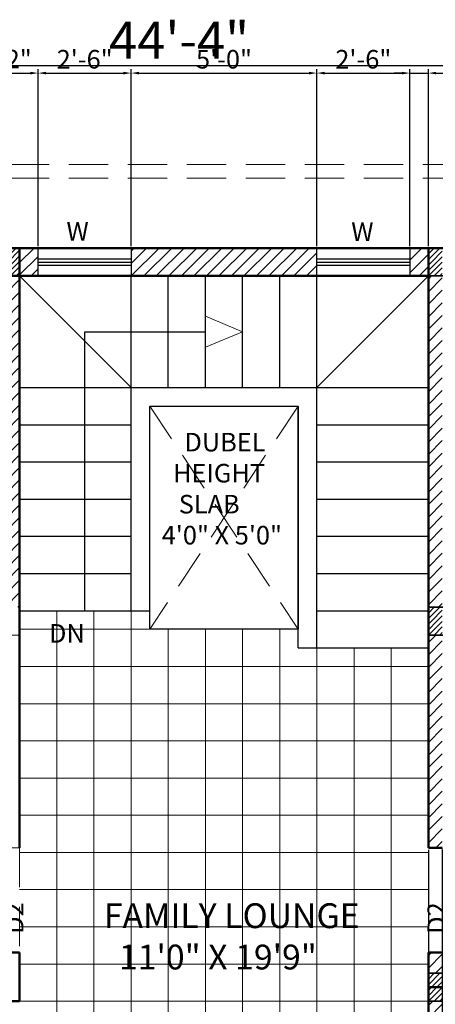
# Model space of a CAD drawing. Units: millimetres. Extents: x 225995 to 227247, y 225507 to 226008.
# Tile 17 of 23: x 226894 to 227029, y 225691 to 226008. Entities that reach past the tile are written whole.
import ezdxf

# ---------------------------------------------------------------- set-up
doc = ezdxf.new("R2010")
doc.units = ezdxf.units.MM
doc.linetypes.add('DASHED', pattern=[19.05, 12.7, -6.35])
for name, color, linetype, lineweight in [('A-ANNO-DIMS', 2, 'Continuous', 18), ('A-ANNO-TEXT', 3, 'Continuous', 18), ('A-AREA-IDEN', 30, 'Continuous', 18), ('A-COLS', 40, 'Continuous', 35), ('A-FLOR-PATT', 8, 'Continuous', 13), ('A-FLOR-STRS', 141, 'Continuous', 25), ('A-FURN', 9, 'Continuous', 18), ('A-GLAZ', 4, 'Continuous', 25), ('A-WALL', 7, 'Continuous', 50), ('A-WALL-OVHD', 1, 'DASHED', 18), ('A-WALL-PATT', 8, 'Continuous', 13)]:
    doc.layers.add(name, color=color, linetype=linetype, lineweight=lineweight)
doc.styles.get("Standard").update_dxf_attribs({"font": 'arial.ttf'})
doc.dimstyles.new('ISO-25', dxfattribs={"dimtxt": 6, "dimasz": 2.5, "dimexe": 1.25, "dimexo": 0.625, "dimtad": 1, "dimdec": 0, "dimlunit": 3, "dimtxsty": 'Standard', "dimcen": 2.5, "dimadec": 0, "dimazin": 0, "dimtfac": 1, "dimtdec": 0, "dimtmove": 0, "dimatfit": 3, "dimfxl": 1, "dimarcsym": 0})
pattern_1 = [(45, (646.0463, 0.931), (-2.020557627, 2.020557627), [])]
pattern_2 = [(45, (646.0463, 0.931), (-0.898025612, 0.898025612), [])]
pattern_3 = [(45, (646.0463, 119.0672), (-0.898025612, 0.898025612), [])]
pattern_4 = [(45, (646.0463, 234.931), (-0.898025612, 0.898025612), [])]
pattern_5 = [(45, (502.0463, 234.931), (-0.898025612, 0.898025612), [])]

# ---------------------------------------------------------------- blocks, each defined once
blk = doc.blocks.new('*D70')
at = {"layer": 'A-ANNO-DIMS', "color": 0, "lineweight": -2, "transparency": 16777216}
for p, q in [((226679.92, 225962.33), (226679.92, 225994.83)), ((227211.92, 225962.33), (227211.92, 225994.83)), ((226682.42, 225993.58), (227209.42, 225993.58))]:
    blk.add_line(p, q, dxfattribs=at)
at = {"layer": 'A-ANNO-DIMS', "color": 0, "transparency": 16777216}
for points in [[(226682.42, 225993.99), (226682.42, 225993.16), (226679.92, 225993.58)], [(227209.42, 225993.99), (227209.42, 225993.16), (227211.92, 225993.58)]]:
    blk.add_solid(points, dxfattribs=at)
at = {"layer": 'Defpoints', "color": 0, "transparency": 16777216}
for p in [(227211.92, 225993.58), (226679.92, 225961.7), (227211.92, 225961.7)]:
    blk.add_point(p, dxfattribs=at)
at = {"layer": 'A-ANNO-DIMS', "color": 0, "transparency": 16777216, "insert": (226945.92, 226000.2), "char_height": 12, "attachment_point": 5}
blk.add_mtext('44\'-4"', dxfattribs=at)
blk = doc.blocks.new('*D115')
at = {"layer": 'A-ANNO-DIMS', "color": 0, "lineweight": -2, "transparency": 16777216}
for p, q in [((227026.42, 225740.58), (227026.42, 225520)), ((227030.92, 225740.58), (227030.92, 225520)), ((227023.92, 225521.25), (227021.42, 225521.25)), ((227026.42, 225521.25), (227030.92, 225521.25)), ((227033.42, 225521.25), (227067.1, 225521.25))]:
    blk.add_line(p, q, dxfattribs=at)
at = {"layer": 'A-ANNO-DIMS', "color": 0, "transparency": 16777216}
for points in [[(227023.92, 225521.67), (227023.92, 225520.84), (227026.42, 225521.25)], [(227033.42, 225521.67), (227033.42, 225520.84), (227030.92, 225521.25)]]:
    blk.add_solid(points, dxfattribs=at)
at = {"layer": 'Defpoints', "color": 0, "transparency": 16777216}
for p in [(227026.42, 225741.2), (227030.92, 225741.2), (227030.92, 225521.25)]:
    blk.add_point(p, dxfattribs=at)
at = {"layer": 'A-ANNO-DIMS', "color": 0, "transparency": 16777216, "insert": (227051.51, 225524.98), "char_height": 6, "attachment_point": 5}
blk.add_mtext('0\'-4 1/2"', dxfattribs=at)
blk = doc.blocks.new('*D117')
at = {"layer": 'A-ANNO-DIMS', "color": 0, "lineweight": -2, "transparency": 16777216}
for p, q in [((226864.05, 225935.33), (226864.05, 225992.4)), ((226866.55, 225991.15), (226897.92, 225991.15)), ((226900.42, 225935.33), (226900.42, 225992.4))]:
    blk.add_line(p, q, dxfattribs=at)
at = {"layer": 'A-ANNO-DIMS', "color": 0, "transparency": 16777216}
for points in [[(226866.55, 225991.57), (226866.55, 225990.74), (226864.05, 225991.15)], [(226897.92, 225991.57), (226897.92, 225990.74), (226900.42, 225991.15)]]:
    blk.add_solid(points, dxfattribs=at)
at = {"layer": 'Defpoints', "color": 0, "transparency": 16777216}
for p in [(226900.42, 225991.15), (226864.05, 225934.7), (226900.42, 225934.7)]:
    blk.add_point(p, dxfattribs=at)
at = {"layer": 'A-ANNO-DIMS', "color": 0, "transparency": 16777216, "insert": (226882.23, 225994.88), "char_height": 6, "attachment_point": 5}
blk.add_mtext('3\'-0 1/2"', dxfattribs=at)
blk = doc.blocks.new('*D118')
at = {"layer": 'A-ANNO-DIMS', "color": 0, "lineweight": -2, "transparency": 16777216}
for p, q in [((226900.42, 225935.33), (226900.42, 225992.4)), ((226902.92, 225991.15), (226927.92, 225991.15)), ((226930.42, 225935.33), (226930.42, 225992.4))]:
    blk.add_line(p, q, dxfattribs=at)
at = {"layer": 'A-ANNO-DIMS', "color": 0, "transparency": 16777216}
for points in [[(226902.92, 225991.57), (226902.92, 225990.74), (226900.42, 225991.15)], [(226927.92, 225991.57), (226927.92, 225990.74), (226930.42, 225991.15)]]:
    blk.add_solid(points, dxfattribs=at)
at = {"layer": 'Defpoints', "color": 0, "transparency": 16777216}
for p in [(226930.42, 225991.15), (226900.42, 225934.7), (226930.42, 225934.7)]:
    blk.add_point(p, dxfattribs=at)
at = {"layer": 'A-ANNO-DIMS', "color": 0, "transparency": 16777216, "insert": (226915.42, 225994.84), "char_height": 6, "attachment_point": 5}
blk.add_mtext('2\'-6"', dxfattribs=at)
blk = doc.blocks.new('*D119')
at = {"layer": 'A-ANNO-DIMS', "color": 0, "lineweight": -2, "transparency": 16777216}
for p, q in [((226930.42, 225935.33), (226930.42, 225992.4)), ((226932.92, 225991.15), (226987.92, 225991.15)), ((226990.42, 225935.33), (226990.42, 225992.4))]:
    blk.add_line(p, q, dxfattribs=at)
at = {"layer": 'A-ANNO-DIMS', "color": 0, "transparency": 16777216}
for points in [[(226932.92, 225991.57), (226932.92, 225990.74), (226930.42, 225991.15)], [(226987.92, 225991.57), (226987.92, 225990.74), (226990.42, 225991.15)]]:
    blk.add_solid(points, dxfattribs=at)
at = {"layer": 'Defpoints', "color": 0, "transparency": 16777216}
for p in [(226990.42, 225991.15), (226930.42, 225934.7), (226990.42, 225934.7)]:
    blk.add_point(p, dxfattribs=at)
at = {"layer": 'A-ANNO-DIMS', "color": 0, "transparency": 16777216, "insert": (226960.42, 225994.84), "char_height": 6, "attachment_point": 5}
blk.add_mtext('5\'-0"', dxfattribs=at)
blk = doc.blocks.new('*D120')
at = {"layer": 'A-ANNO-DIMS', "color": 0, "lineweight": -2, "transparency": 16777216}
for p, q in [((226990.42, 225935.33), (226990.42, 225992.4)), ((226992.92, 225991.15), (227017.92, 225991.15)), ((227020.42, 225935.33), (227020.42, 225992.4))]:
    blk.add_line(p, q, dxfattribs=at)
at = {"layer": 'A-ANNO-DIMS', "color": 0, "transparency": 16777216}
for points in [[(226992.92, 225991.57), (226992.92, 225990.74), (226990.42, 225991.15)], [(227017.92, 225991.57), (227017.92, 225990.74), (227020.42, 225991.15)]]:
    blk.add_solid(points, dxfattribs=at)
at = {"layer": 'Defpoints', "color": 0, "transparency": 16777216}
for p in [(227020.42, 225991.15), (226990.42, 225934.7), (227020.42, 225934.7)]:
    blk.add_point(p, dxfattribs=at)
at = {"layer": 'A-ANNO-DIMS', "color": 0, "transparency": 16777216, "insert": (227005.42, 225994.84), "char_height": 6, "attachment_point": 5}
blk.add_mtext('2\'-6"', dxfattribs=at)
blk = doc.blocks.new('*D121')
at = {"layer": 'A-ANNO-DIMS', "color": 0, "lineweight": -2, "transparency": 16777216}
for p, q in [((227017.92, 225991.15), (227015.42, 225991.15)), ((227020.42, 225935.33), (227020.42, 225992.4)), ((227020.42, 225991.15), (227026.42, 225991.15)), ((227026.42, 225935.33), (227026.42, 225992.4)), ((227028.92, 225991.15), (227048.62, 225991.15))]:
    blk.add_line(p, q, dxfattribs=at)
at = {"layer": 'A-ANNO-DIMS', "color": 0, "transparency": 16777216}
for points in [[(227017.92, 225991.57), (227017.92, 225990.74), (227020.42, 225991.15)], [(227028.92, 225991.57), (227028.92, 225990.74), (227026.42, 225991.15)]]:
    blk.add_solid(points, dxfattribs=at)
at = {"layer": 'Defpoints', "color": 0, "transparency": 16777216}
for p in [(227026.42, 225991.15), (227020.42, 225934.7), (227026.42, 225934.7)]:
    blk.add_point(p, dxfattribs=at)
at = {"layer": 'A-ANNO-DIMS', "color": 0, "transparency": 16777216, "insert": (227040.02, 225994.84), "char_height": 6, "attachment_point": 5}
blk.add_mtext('0\'-6"', dxfattribs=at)

msp = doc.modelspace()

# ---------------------------------------------------------------- hatches: boundary and pattern name
at = {"layer": 'A-WALL-PATT'}
h = msp.add_hatch(dxfattribs=at)
h.set_pattern_fill('ANSI31', color=256, scale=0.4)
h.set_pattern_definition(pattern_5)
h.paths.add_polyline_path([(226894.42, 225934.7), (226886.92, 225934.7), (226886.92, 225930.2), (226894.42, 225930.2)])
h = msp.add_hatch(dxfattribs=at)
h.set_pattern_fill('ANSI31', color=256, scale=0.9)
h.set_pattern_definition(pattern_1)
h.paths.add_polyline_path([(226900.42, 225934.7), (226894.42, 225934.7), (226894.42, 225925.7), (226900.42, 225925.7)])
h = msp.add_hatch(dxfattribs=at)
h.set_pattern_fill('ANSI31', color=256, scale=0.9)
h.set_pattern_definition(pattern_1)
h.paths.add_polyline_path([(226990.42, 225934.7), (226930.42, 225934.7), (226930.42, 225925.7), (226990.42, 225925.7)])
h = msp.add_hatch(dxfattribs=at)
h.set_pattern_fill('ANSI31', color=256, scale=0.9)
h.set_pattern_definition(pattern_1)
h.paths.add_polyline_path([(227026.42, 225934.7), (227020.42, 225934.7), (227020.42, 225925.7), (227026.42, 225925.7)])
h = msp.add_hatch(dxfattribs=at)
h.set_pattern_fill('ANSI31', color=256, scale=0.4)
h.set_pattern_definition(pattern_4)
h.paths.add_polyline_path([(227030.92, 225934.7), (227026.42, 225934.7), (227026.42, 225930.2), (227030.92, 225930.2)])
h = msp.add_hatch(dxfattribs=at)
h.set_pattern_fill('ANSI31', color=256, scale=0.4)
h.set_pattern_definition(pattern_5)
h.paths.add_polyline_path([(226894.42, 225930.2), (226886.92, 225930.2), (226886.92, 225925.7), (226894.42, 225925.7)])
h = msp.add_hatch(dxfattribs=at)
h.set_pattern_fill('ANSI31', color=256, scale=0.4)
h.set_pattern_definition(pattern_4)
h.paths.add_polyline_path([(227030.92, 225930.2), (227026.42, 225930.2), (227026.42, 225925.7), (227030.92, 225925.7)])
h = msp.add_hatch(dxfattribs=at)
h.set_pattern_fill('ANSI31', color=256, scale=0.9)
h.paths.add_polyline_path([(226894.42, 225925.7), (226889.92, 225925.7), (226889.92, 225818.84), (226894.42, 225818.84)])
h = msp.add_hatch(dxfattribs=at)
h.set_pattern_fill('ANSI31', color=256, scale=0.9)
h.set_pattern_definition(pattern_1)
h.paths.add_polyline_path([(227030.92, 225925.7), (227026.42, 225925.7), (227026.42, 225818.84), (227030.92, 225818.84)])
h = msp.add_hatch(dxfattribs=at)
h.set_pattern_fill('ANSI31', color=256, scale=0.4)
h.set_pattern_definition(pattern_3)
h.paths.add_polyline_path([(227030.92, 225818.84), (227026.42, 225818.84), (227026.42, 225814.34), (227030.92, 225814.34)])
h = msp.add_hatch(dxfattribs=at)
h.set_pattern_fill('ANSI31', color=256, scale=0.4)
h.set_pattern_definition(pattern_3)
h.paths.add_polyline_path([(227030.92, 225814.34), (227026.42, 225814.34), (227026.42, 225809.84), (227030.92, 225809.84)])
h = msp.add_hatch(dxfattribs=at)
h.set_pattern_fill('ANSI31', color=256, scale=0.9)
h.set_pattern_definition(pattern_1)
h.paths.add_polyline_path([(227030.92, 225809.84), (227026.42, 225809.84), (227026.42, 225741.2), (227030.92, 225741.2)])
h = msp.add_hatch(dxfattribs=at)
h.set_pattern_fill('ANSI31', color=256, scale=0.9)
h.set_pattern_definition(pattern_1)
h.paths.add_polyline_path([(227030.92, 225707.45), (227026.42, 225707.45), (227026.42, 225700.7), (227030.92, 225700.7)])
h = msp.add_hatch(dxfattribs=at)
h.set_pattern_fill('ANSI31', color=256, scale=0.4)
h.set_pattern_definition(pattern_2)
h.paths.add_polyline_path([(227030.92, 225700.7), (227026.42, 225700.7), (227026.42, 225696.2), (227030.92, 225696.2)])
h = msp.add_hatch(dxfattribs=at)
h.set_pattern_fill('ANSI31', color=256, scale=0.4)
h.set_pattern_definition(pattern_2)
h.paths.add_polyline_path([(227030.92, 225696.2), (227026.42, 225696.2), (227026.42, 225691.7), (227030.92, 225691.7)])
h = msp.add_hatch(dxfattribs=at)
h.set_pattern_fill('ANSI31', color=256, scale=0.9)
h.set_pattern_definition(pattern_1)
h.paths.add_polyline_path([(227030.92, 225691.7), (227026.42, 225691.7), (227026.42, 225580.7), (227030.92, 225580.7)])

# ---------------------------------------------------------------- linework, layer by layer
at = {"layer": 'A-COLS'}
for points in [[(226882.42, 225925.7), (226882.42, 225934.7), (226894.42, 225934.7), (226894.42, 225925.7)], [(227026.42, 225925.7), (227026.42, 225934.7), (227038.42, 225934.7), (227038.42, 225925.7)], [(227026.42, 225809.84), (227026.42, 225818.84), (227038.42, 225818.84), (227038.42, 225809.84)], [(227026.42, 225691.7), (227026.42, 225700.7), (227038.42, 225700.7), (227038.42, 225691.7)]]:
    msp.add_lwpolyline(points, close=True, dxfattribs=at)
at = {"layer": 'A-FLOR-PATT'}
for p, q in [((226906.42, 225580.7), (226906.42, 225817.7)), ((226918.42, 225580.7), (226918.42, 225817.7)), ((226918.42, 225580.7), (226918.42, 225817.7)), ((226930.42, 225580.7), (226930.42, 225817.7)), ((226990.42, 225578.36), (226990.42, 225817.7)), ((226894.42, 225811.7), (226984.42, 225811.7)), ((226942.42, 225578.36), (226942.42, 225811.7)), ((226954.42, 225580.7), (226954.42, 225811.7)), ((226966.42, 225580.7), (226966.42, 225811.7)), ((226978.42, 225580.7), (226978.42, 225811.7)), ((227002.42, 225580.7), (227002.42, 225805.7)), ((227014.42, 225580.7), (227014.42, 225805.7)), ((226894.42, 225799.7), (227026.42, 225799.7)), ((226894.42, 225787.7), (227026.42, 225787.7)), ((226894.42, 225775.7), (227026.42, 225775.7)), ((226894.42, 225763.7), (227026.42, 225763.7)), ((226894.42, 225751.7), (227026.42, 225751.7)), ((226894.42, 225739.7), (227026.42, 225739.7)), ((226894.42, 225727.7), (227026.42, 225727.7)), ((226894.42, 225715.7), (227026.42, 225715.7)), ((226894.42, 225703.7), (227026.42, 225703.7)), ((226894.42, 225691.7), (227026.42, 225691.7))]:
    msp.add_line(p, q, dxfattribs=at)
at = {"layer": 'A-FLOR-STRS'}
for p, q in [((226894.42, 225925.7), (226930.42, 225889.7)), ((226930.42, 225817.7), (226930.42, 225925.7)), ((226942.42, 225889.7), (226942.42, 225925.7)), ((226954.42, 225889.7), (226954.42, 225925.7)), ((226966.42, 225889.7), (226966.42, 225925.7)), ((226978.42, 225889.7), (226978.42, 225925.7)), ((226990.42, 225805.7), (226990.42, 225925.7)), ((226990.42, 225889.7), (227026.42, 225925.7)), ((226915.42, 225817.7), (226915.42, 225907.7)), ((226915.42, 225907.7), (226954.42, 225907.7)), ((226894.42, 225889.7), (227026.42, 225889.7)), ((226936.42, 225883.7), (226984.42, 225883.7)), ((226936.42, 225817.7), (226936.42, 225883.7)), ((226984.42, 225805.7), (226984.42, 225883.7)), ((226894.42, 225877.7), (226930.42, 225877.7)), ((226990.42, 225877.7), (227026.42, 225877.7)), ((226894.42, 225865.7), (226930.42, 225865.7)), ((226990.42, 225865.7), (227026.42, 225865.7)), ((226894.42, 225853.7), (226930.42, 225853.7)), ((226990.42, 225853.7), (227026.42, 225853.7)), ((226894.42, 225841.7), (226930.42, 225841.7)), ((226990.42, 225841.7), (227026.42, 225841.7)), ((226894.42, 225829.7), (226930.42, 225829.7)), ((226990.42, 225829.7), (227026.42, 225829.7)), ((226894.42, 225817.7), (226936.42, 225817.7)), ((226990.42, 225817.7), (227026.42, 225817.7)), ((226984.42, 225805.7), (227026.42, 225805.7))]:
    msp.add_line(p, q, dxfattribs=at)
msp.add_lwpolyline([(226936.42, 225883.7), (226984.42, 225883.7), (226984.42, 225811.7), (226936.42, 225811.7)], close=True, dxfattribs=at)
at = {"layer": 'A-FURN'}
for p, q in [((226900.42, 225934.7), (226900.42, 225925.7)), ((226930.42, 225934.7), (226930.42, 225925.7)), ((226990.42, 225934.7), (226990.42, 225925.7)), ((227020.42, 225934.7), (227020.42, 225925.7)), ((226966.42, 225907.7), (226954.42, 225912.68)), ((226954.42, 225912.68), (226954.42, 225902.73)), ((226966.42, 225907.7), (226954.42, 225902.73)), ((226889.92, 225809.85), (226894.42, 225809.84))]:
    msp.add_line(p, q, dxfattribs=at)
at = {"layer": 'A-GLAZ'}
for p, q in [((226900.42, 225931.2), (226930.42, 225931.2)), ((226990.42, 225931.2), (227020.42, 225931.2)), ((226900.42, 225930.2), (226930.42, 225930.2)), ((226900.42, 225929.2), (226930.42, 225929.2)), ((226990.42, 225929.2), (227020.42, 225929.2)), ((226990.48, 225930.2), (227020.42, 225930.2))]:
    msp.add_line(p, q, dxfattribs=at)
for points in [[(226900.42, 225934.7), (226930.42, 225934.7), (226930.42, 225925.7), (226900.42, 225925.7)], [(226990.42, 225934.7), (227020.42, 225934.7), (227020.42, 225925.7), (226990.42, 225925.7)]]:
    msp.add_lwpolyline(points, close=True, dxfattribs=at)
at = {"layer": 'A-WALL'}
for p, q in [((226757.92, 225934.7), (227211.92, 225934.7)), ((226757.92, 225934.7), (227211.92, 225934.7)), ((226894.42, 225934.7), (226894.42, 225925.7)), ((227026.42, 225934.7), (227026.42, 225925.7)), ((226757.92, 225925.7), (227026.42, 225925.7)), ((226894.42, 225741.2), (226894.42, 225925.7)), ((227026.42, 225925.7), (226894.42, 225925.7)), ((227026.42, 225741.2), (227026.42, 225925.7)), ((227026.42, 225741.2), (227026.42, 225925.7)), ((227026.42, 225741.2), (227030.92, 225741.2)), ((227030.92, 225741.2), (227026.42, 225741.2)), ((226889.92, 225707.45), (226894.42, 225707.45)), ((226889.92, 225707.45), (226894.42, 225707.45)), ((226894.42, 225691.7), (226894.42, 225707.45)), ((226894.42, 225707.45), (226894.42, 225700.7)), ((227026.42, 225580.7), (227026.42, 225707.45)), ((227026.42, 225707.45), (227030.92, 225707.45)), ((227026.42, 225580.7), (227026.42, 225707.45)), ((227026.42, 225707.45), (227030.92, 225707.45)), ((226894.42, 225700.7), (226894.42, 225691.7)), ((227026.42, 225696.2), (227057.92, 225696.2)), ((226894.42, 225691.7), (226889.92, 225691.7))]:
    msp.add_line(p, q, dxfattribs=at)
at = {"layer": 'A-WALL-OVHD'}
for p, q in [((226757.92, 225961.7), (227211.92, 225961.7)), ((226757.92, 225957.2), (227207.42, 225957.2)), ((226936.42, 225883.7), (226984.42, 225811.7)), ((226984.42, 225883.7), (226936.42, 225811.7))]:
    msp.add_line(p, q, dxfattribs=at)
for points in [[(226889.92, 225741.2), (226894.42, 225741.2), (226894.42, 225707.45), (226889.92, 225707.45)], [(227026.42, 225741.2), (227030.92, 225741.2), (227030.92, 225707.45), (227026.42, 225707.45)]]:
    msp.add_lwpolyline(points, close=True, dxfattribs=at)

# ---------------------------------------------------------------- texts
at = {"layer": 'A-ANNO-TEXT', "char_height": 6, "attachment_point": 1}
for s, insert in [('   W', (226904.03, 225943.09)), ('   W', (226996.02, 225942.96)), ('   DN', (226898.39, 225813.38))]:
    msp.add_mtext_dynamic_manual_height_columns(s, width=24.8115, gutter_width=12.5, heights=[0], dxfattribs=dict(at, insert=insert))
at = {"layer": 'A-ANNO-TEXT', "char_height": 6, "attachment_point": 1, "rotation": 90}
for insert in [(226889.64, 225713.45), (227026.14, 225713.45)]:
    msp.add_mtext_dynamic_manual_height_columns('D2', width=8.157, gutter_width=12.5, heights=[0], dxfattribs=dict(at, insert=insert))
at = {"layer": 'A-AREA-IDEN', "attachment_point": 1}
for s, width, insert, char_height in [('      DUBEL\\P    HEIGHT\\P     SLAB\\P  4\'0" X 5\'0"', 85.4795, (226936.64, 225875.07), 6), (' FAMILY LOUNGE\\P   11\'0" X 19\'9"', 95.6826, (226919.16, 225723.29), 8)]:
    msp.add_mtext_dynamic_manual_height_columns(s, width=width, gutter_width=12.5, heights=[0], dxfattribs=dict(at, insert=insert, char_height=char_height))

# ---------------------------------------------------------------- dimensions: what is measured, and where the dimension line sits
at = {"layer": 'A-ANNO-DIMS'}
for base, p1, p2, override, picture, middle in [((227211.92, 225993.58), (226679.92, 225961.7), (227211.92, 225961.7), {"dimtxt": 12, "dimclrd": 0, "dimclre": 0, "dimclrt": 0}, '*D70', (226945.92, 226000.2)), ((226900.42, 225991.15), (226864.05, 225934.7), (226900.42, 225934.7), {"dimdec": 1, "dimlfac": 1, "dimrnd": 0, "dimzin": 1, "dimdsep": 46, "dimlunit": 4, "dimfrac": 2}, '*D117', (226882.23, 225994.88)), ((226930.42, 225991.15), (226900.42, 225934.7), (226930.42, 225934.7), {"dimdec": 1, "dimlfac": 1, "dimrnd": 0, "dimzin": 1, "dimdsep": 46, "dimlunit": 4, "dimfrac": 2}, '*D118', (226915.42, 225994.84)), ((226990.42, 225991.15), (226930.42, 225934.7), (226990.42, 225934.7), {"dimdec": 1, "dimlfac": 1, "dimrnd": 0, "dimzin": 1, "dimdsep": 46, "dimlunit": 4, "dimfrac": 2}, '*D119', (226960.42, 225994.84)), ((227020.42, 225991.15), (226990.42, 225934.7), (227020.42, 225934.7), {"dimdec": 1, "dimlfac": 1, "dimrnd": 0, "dimzin": 1, "dimdsep": 46, "dimlunit": 4, "dimfrac": 2}, '*D120', (227005.42, 225994.84)), ((227026.42, 225991.15), (227020.42, 225934.7), (227026.42, 225934.7), {"dimdec": 1, "dimlfac": 1, "dimrnd": 0, "dimzin": 1, "dimdsep": 46, "dimlunit": 4, "dimfrac": 2}, '*D121', (227040.02, 225994.84)), ((227030.92, 225521.25), (227026.42, 225741.2), (227030.92, 225741.2), {"dimdec": 1, "dimlfac": 1, "dimrnd": 0, "dimzin": 1, "dimdsep": 46, "dimlunit": 4, "dimfrac": 2}, '*D115', (227051.51, 225524.98))]:
    dim = msp.add_linear_dim(base=base, p1=p1, p2=p2, dimstyle='ISO-25', override=override, dxfattribs=at)
    dim.commit()
    dim.dimension.update_dxf_attribs({"geometry": picture, "text_midpoint": middle})

doc.saveas('drawing.dxf')
